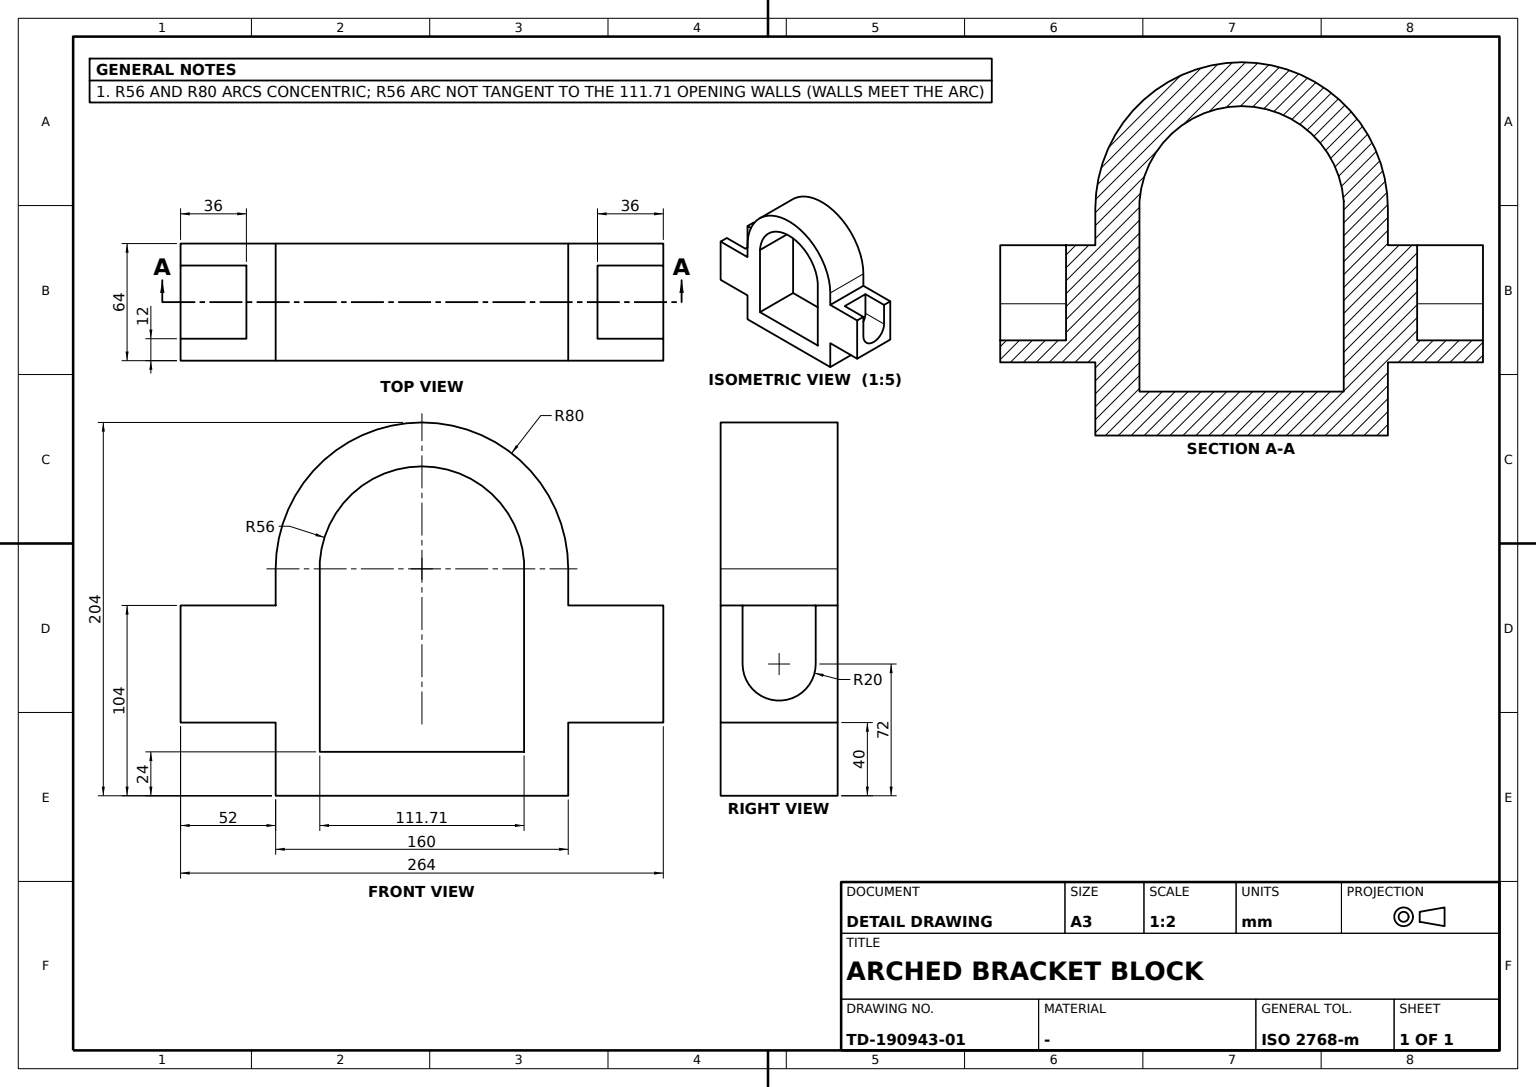
CATIA V5 part; units mm, degrees
sketch "Sketch1" plane through (0, 0, 0) normal (1, 0, 0) x (0, 1, 0)
  arc A0 (80, 0) -> (-80, 0) centre (0, 0) ccw
  arc A1 (55.857, 4) -> (-55.857, 4) centre (0, 0) ccw
  point P0 (-80, 0)
  line L0 (-80, 0) -> (-80, -20)
  point P1 (-80, -124)
  line L1 (-80, -124) -> (80, -124)
  line L2 (80, -124) -> (80, -84)
  point P2 (80, 0)
  line L3 (-55.857, 4) -> (-55.857, -100)
  line L4 (-55.857, -100) -> (55.857, -100)
  line L5 (55.857, -100) -> (55.857, 4)
  line L6 (55.857, 0) -> (56, 0) construction
  point P3 (55.857, 0)
  point P4 (-55.857, 0)
  line L7 (-56, 0) -> (-55.857, 0) construction
  point P5 (-56, 0)
  point P6 (-80, -20)
  line L8 (-80, -20) -> (-132, -20)
  point P7 (-132, -20)
  line L9 (-132, -20) -> (-132, -84)
  point P8 (-132, -84)
  line L10 (-132, -84) -> (-80, -84)
  point P9 (-80, -84)
  point P10 (132, -20)
  point P11 (80, -20)
  line L11 (80, -20) -> (132, -20)
  point P12 (132, -84)
  line L12 (132, -20) -> (132, -84)
  point P13 (80, -84)
  line L13 (132, -84) -> (80, -84)
  line L14 (-80, -84) -> (-80, -124)
  line L15 (80, -20) -> (80, 0)
  dimension "radius A1" = 56
  dimension "length L1" = 160
  dimension "distance L4 L1" = 24
  dimension "distance L1 origin" = 124
  dimension "length L5" = 104
  dimension "length L9" = 64
  dimension "distance L10 P1" = 40
  dimension "length L10" = 52
  constraint coincidence P0 x-axis
  constraint coincidence P2 x-axis
  constraint coincidence L5 P3
  constraint coincidence L3 P4
  constraint coincidence A1 P5
  constraint coincidence P9 L0
  constraint coincidence L0 L14
  constraint coincidence L2 L15
  constraint vertical L0 y-axis
  constraint vertical L2 y-axis
  constraint vertical L3 y-axis
  constraint vertical L5 y-axis
  constraint vertical L9 y-axis
  constraint vertical L14 y-axis
  constraint vertical L15 y-axis
  constraint horizontal L1 x-axis
  constraint horizontal L4 x-axis
  constraint horizontal L6 x-axis
  constraint horizontal L7 x-axis
  constraint horizontal L8 x-axis
  constraint horizontal L10 x-axis
  constraint symmetry L0 L2 y-axis
  constraint symmetry L3 L5 y-axis
  constraint symmetry P7 P10 y-axis
  constraint symmetry P6 P11 y-axis
  constraint symmetry L8 L11 y-axis
  constraint symmetry P8 P12 y-axis
  constraint symmetry L9 L12 y-axis
  constraint symmetry P9 P13 y-axis
  constraint symmetry L10 L13 y-axis
extrude "Pad1" add sketch "Sketch1" along normal mid plane 64
sketch "Sketch2" plane through (0, 132, 0) normal (0, 1, 0) x (-1, 0, 0)
  arc A0 (-20, -52) -> (20, -52) centre (0, -52) ccw
  point P0 (0, -52)
  point P1 (20, -52)
  line L0 (20, -52) -> (20, -20)
  line L1 (20, -20) -> (-20, -20)
  line L2 (-20, -20) -> (-20, -52)
  point P2 (-20, -52)
  line L3 (32, -84) -> (-32, -84) construction
  line L4 (32, -20) -> (-32, -20) construction
  point P3 (-20, -52)
  point P4 (20, -52)
  dimension "radius A0" = 20
  dimension "distance P0 L3" = 32
  dimension "length L0" = 32
  constraint coincidence P0 y-axis
  constraint coincidence P2 A0
  constraint coincidence P1 A0
  constraint coincidence L1 L4
  constraint coincidence L0 P4
  constraint coincidence L2 P3
  constraint coincidence P1 P4
  constraint coincidence P2 P3
  constraint vertical L0 y-axis
  constraint vertical L2 y-axis
  constraint horizontal L1 x-axis
  constraint symmetry L0 L2 y-axis
extrude "Pocket1" cut sketch "Sketch2" against normal blind 36
mirror "Mirror1" about plane through (0, 0, 0) normal (0, 1, 0) of "Pocket1"
